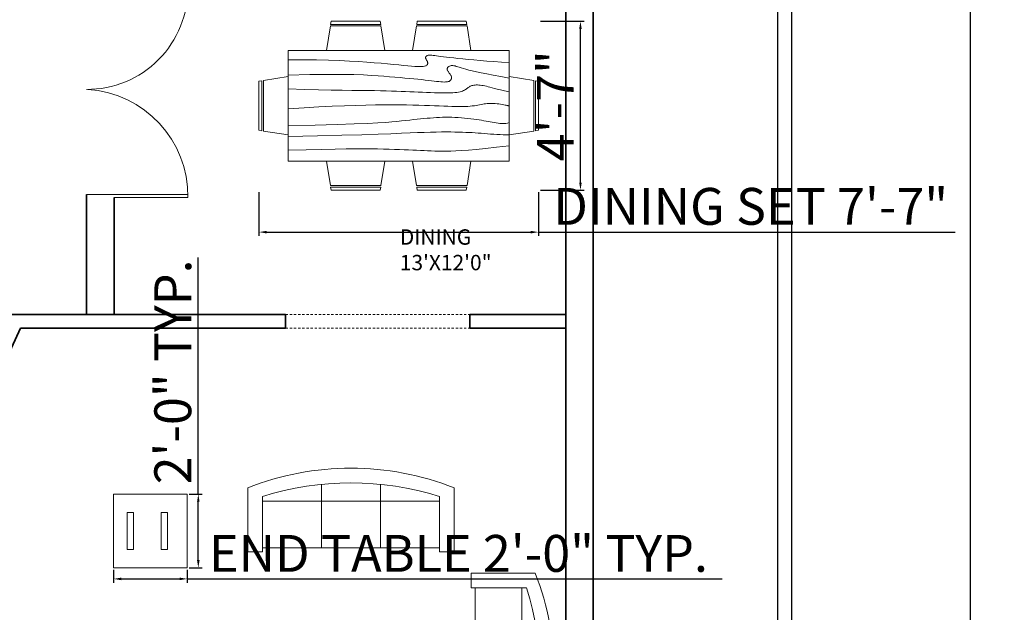
# Model space of a CAD drawing. Units: inches. Extents: x 2562 to 3392, y 1021 to 2243.
# Tile 4 of 6: x 2986 to 3306, y 1472 to 1665. Entities that reach past the tile are written whole.
import ezdxf

# ---------------------------------------------------------------- set-up
doc = ezdxf.new("R2010")
doc.units = ezdxf.units.IN
doc.linetypes.add('JIS_02_0.7', pattern=[1.35, 0.75, -0.6])
for name, color, linetype, lineweight in [('A-ANNO-DIMS', 2, 'Continuous', 18), ('A-AREA-IDEN', 7, 'Continuous', 18), ('A-DOOR', 4, 'Continuous', 18), ('A-FURN', 8, 'Continuous', 18), ('A-WALL', 7, 'Continuous', 35), ('A-WALL-HIDN', 7, 'JIS_02_0.7', 18), ('C-PROP', 7, 'Continuous', 30)]:
    doc.layers.add(name, color=color, linetype=linetype, lineweight=lineweight)
doc.styles.get("Standard").update_dxf_attribs({"font": 'arial.ttf'})
doc.dimstyles.new('ISO-25', dxfattribs={"dimtxt": 12, "dimasz": 2.5, "dimexe": 1.25, "dimexo": 0.625, "dimtad": 1, "dimdec": 1, "dimlunit": 3, "dimtxsty": 'Standard', "dimcen": 2.5, "dimadec": 0, "dimazin": 0, "dimtfac": 1, "dimtdec": 1, "dimtmove": 0, "dimatfit": 3, "dimfxl": 1, "dimarcsym": 0})

# ---------------------------------------------------------------- blocks, each defined once
blk = doc.blocks.new('Dining Set - 36 x 72 in.')
for p, q in [((-22.2343, 26.00059), (-23.4847, 17.99762)), ((-22.2304, 26), (-5.7608, 26)), ((-22, 27.5), (-22.1562, 26.50042)), ((-5.8416, 26.5), (-22.1534, 26.5)), ((-22, 27.5), (-6, 27.5)), ((-5.8437, 26.49966), (-6, 27.5)), ((-4.5152, 17.99762), (-5.7655, 25.99926)), ((5.7657, 26.00059), (4.5153, 17.99762)), ((5.7696, 26), (22.2392, 26)), ((6, 27.5), (5.8438, 26.50042)), ((22.1584, 26.5), (5.8466, 26.5)), ((6, 27.5), (22, 27.5)), ((22.1563, 26.49966), (22, 27.5)), ((23.4848, 17.99762), (22.2345, 25.99926)), ((36, 18), (-36, 18)), ((-36, 18), (-36, -18)), ((36, -18), (36, 18)), ((-45.5, 8), (-44.5004, 8.15617)), ((-45.5, 8), (-45.5, -8)), ((-44.5, -8.15843), (-44.5, 8.15338)), ((-44.0006, 8.23428), (-35.9976, 9.48474)), ((-44, 8.23041), (-44, -8.23915)), ((44.0006, 8.23428), (35.9976, 9.48474)), ((44, 8.23041), (44, -8.23915)), ((44.5, -8.15843), (44.5, 8.15338)), ((45.5, 8), (44.5005, 8.15617)), ((45.5, 8), (45.5, -8)), ((-44.4997, -8.15631), (-45.5, -8)), ((-35.9976, -9.48476), (-43.9993, -8.2345)), ((35.9976, -9.48476), (43.9993, -8.2345)), ((44.4997, -8.15631), (45.5, -8)), ((-36, -18), (36, -18)), ((-22.2343, -26.0006), (-23.4847, -17.99762)), ((-4.5152, -17.99762), (-5.7655, -25.99928)), ((5.7657, -26.0006), (4.5153, -17.99762)), ((23.4848, -17.99762), (22.2345, -25.99928)), ((-22.2304, -26), (-5.7608, -26)), ((-22, -27.5), (-22.1562, -26.50044)), ((-5.8416, -26.5), (-22.1534, -26.5)), ((-22, -27.5), (-6, -27.5)), ((-5.8437, -26.49967), (-6, -27.5)), ((5.7696, -26), (22.2392, -26)), ((6, -27.5), (5.8438, -26.50044)), ((22.1584, -26.5), (5.8466, -26.5)), ((6, -27.5), (22, -27.5)), ((22.1563, -26.49967), (22, -27.5))]:
    blk.add_line(p, q)
for points in [[(-36, 15), (-31.1772, 14.97754), (-26.8079, 14.91406), (-22.8538, 14.81543), (-19.276, 14.6875), (-16.0362, 14.53613), (-13.0957, 14.36718), (-10.4159, 14.18652), (-7.9583, 14), (-5.6904, 13.81315), (-3.6035, 13.63021), (-1.6954, 13.45508), (0.0365, 13.29166), (1.5945, 13.14388), (2.9811, 13.01562), (4.1988, 12.9108), (5.25, 12.83333), (6.1393, 12.78613), (6.8802, 12.76823), (7.4883, 12.77767), (7.9792, 12.8125), (8.3685, 12.87077), (8.6719, 12.95052), (8.9049, 13.0498), (9.0833, 13.16666), (9.2205, 13.29899), (9.3216, 13.44401), (9.3895, 13.59879), (9.4271, 13.76041), (9.4373, 13.92594), (9.4232, 14.09245), (9.3875, 14.257), (9.3333, 14.41666), (9.2638, 14.56917), (9.1836, 14.71484), (9.0975, 14.85465), (9.0104, 14.98958), (8.9272, 15.1206), (8.8529, 15.2487), (8.7922, 15.37483), (8.75, 15.5), (8.7305, 15.62467), (8.7344, 15.74739), (8.7617, 15.86621), (8.8125, 15.97916), (8.8867, 16.08431), (8.9844, 16.17968), (9.1055, 16.26334), (9.25, 16.33333), (9.4189, 16.38802), (9.6172, 16.42708), (9.8506, 16.45052), (10.125, 16.45833), (10.4463, 16.45052), (10.8203, 16.42708), (11.2529, 16.38802), (11.75, 16.33333), (12.3184, 16.26318), (12.9694, 16.17838), (13.7151, 16.07991), (14.5677, 15.96875), (15.5395, 15.84586), (16.6426, 15.71224), (17.8893, 15.56884), (19.2917, 15.41666), (20.859, 15.25667), (22.5879, 15.08984), (24.4721, 14.91715), (26.5052, 14.73958), (28.6809, 14.5581), (30.9929, 14.3737), (33.4347, 14.18733), (36, 14)], [(-36, 10), (-28.9766, 10.14274), (-23.1725, 10.20442), (-18.4241, 10.19775), (-14.5677, 10.13541), (-11.4399, 10.03011), (-8.877, 9.89453), (-6.7154, 9.74137), (-4.7917, 9.58333), (-2.9698, 9.43082), (-1.2246, 9.28515), (0.4415, 9.14534), (2.026, 9.01041), (3.5266, 8.87939), (4.9408, 8.7513), (6.266, 8.62516), (7.5, 8.5), (8.6411, 8.37549), (9.6914, 8.2539), (10.6538, 8.13818), (11.5312, 8.03125), (12.3267, 7.93603), (13.043, 7.85547), (13.6831, 7.79248), (14.25, 7.75), (14.7471, 7.7303), (15.1797, 7.73307), (15.5537, 7.75732), (15.875, 7.80208), (16.1494, 7.86637), (16.3828, 7.94922), (16.5811, 8.04964), (16.75, 8.16666), (16.8944, 8.29915), (17.0143, 8.44531), (17.1089, 8.60319), (17.1771, 8.77083), (17.218, 8.94629), (17.2305, 9.1276), (17.2137, 9.31282), (17.1667, 9.5), (17.0895, 9.6875), (16.987, 9.875), (16.8649, 10.0625), (16.7292, 10.25), (16.5856, 10.4375), (16.4401, 10.625), (16.2985, 10.8125), (16.1667, 11), (16.05, 11.18733), (15.9518, 11.3737), (15.8752, 11.5581), (15.8229, 11.73958), (15.798, 11.91715), (15.8034, 12.08984), (15.842, 12.25667), (15.9167, 12.41666), (16.0295, 12.56836), (16.1784, 12.70833), (16.3605, 12.83268), (16.5729, 12.9375), (16.8127, 13.01888), (17.0768, 13.07291), (17.3625, 13.0957), (17.6667, 13.08333), (17.9894, 13.03312), (18.3418, 12.94726), (18.7382, 12.82918), (19.1927, 12.68229), (19.7195, 12.51001), (20.3327, 12.31575), (21.0465, 12.10294), (21.875, 11.875), (22.8357, 11.63354), (23.959, 11.37304), (25.2786, 11.08618), (26.8282, 10.76562), (28.6414, 10.40405), (30.752, 9.99414), (33.1936, 9.52856), (36, 9)], [(-36, 5.5), (-30.7157, 5.3348), (-26.069, 5.20963), (-21.9946, 5.11767), (-18.4271, 5.05208), (-15.3009, 5.00602), (-12.5508, 4.97265), (-10.1112, 4.94515), (-7.9167, 4.91666), (-5.909, 4.88167), (-4.0586, 4.83984), (-2.3429, 4.79215), (-0.7396, 4.73958), (0.7739, 4.6831), (2.22, 4.6237), (3.6213, 4.56233), (5, 4.5), (6.373, 4.43782), (7.7344, 4.3776), (9.0723, 4.32129), (10.375, 4.27083), (11.6309, 4.22819), (12.8281, 4.19531), (13.9551, 4.17415), (15, 4.16666), (15.954, 4.17448), (16.819, 4.19791), (17.6001, 4.23698), (18.3021, 4.29166), (18.9299, 4.36198), (19.4883, 4.44791), (19.9823, 4.54948), (20.4167, 4.66666), (20.7969, 4.79899), (21.1302, 4.94401), (21.4245, 5.09879), (21.6875, 5.26041), (21.9271, 5.42594), (22.1511, 5.59245), (22.3672, 5.757), (22.5834, 5.91666), (22.8065, 6.06868), (23.0404, 6.21093), (23.2879, 6.34147), (23.5521, 6.45833), (23.8358, 6.55957), (24.142, 6.64323), (24.4735, 6.70735), (24.8334, 6.75), (25.2235, 6.76969), (25.642, 6.76692), (26.0858, 6.74267), (26.5521, 6.69791), (27.0379, 6.63362), (27.5404, 6.55078), (28.0565, 6.45036), (28.5834, 6.33333), (29.1242, 6.19987), (29.7071, 6.04687), (30.3661, 5.87044), (31.1354, 5.66666), (32.0493, 5.43164), (33.142, 5.16146), (34.4475, 4.85221), (36, 4.5)], [(-36, -1), (-30.7915, -0.6591), (-26.0195, -0.38216), (-21.6519, -0.16284), (-17.6563, 0.00521), (-14.0005, 0.12833), (-10.6523, 0.21289), (-7.5796, 0.26522), (-4.75, 0.29166), (-2.134, 0.29793), (0.2878, 0.28711), (2.5317, 0.26163), (4.6146, 0.22396), (6.5529, 0.17651), (8.3633, 0.12174), (10.0623, 0.06209), (11.6667, 0), (13.1899, -0.06201), (14.6341, -0.1211), (15.9982, -0.17432), (17.2813, -0.21875), (18.4823, -0.25147), (19.6003, -0.26953), (20.6343, -0.27002), (21.5834, -0.25), (22.4481, -0.20768), (23.2357, -0.14584), (23.9549, -0.06836), (24.6146, 0.02083), (25.2235, 0.11784), (25.7904, 0.21875), (26.3241, 0.31966), (26.8334, 0.41666), (27.3265, 0.50618), (27.8099, 0.58593), (28.2894, 0.65397), (28.7709, 0.70833), (29.2601, 0.74707), (29.763, 0.76823), (30.2855, 0.76985), (30.8334, 0.75), (31.4088, 0.70784), (31.9994, 0.64713), (32.589, 0.57275), (33.1615, 0.48958), (33.7008, 0.4025), (34.1908, 0.3164), (34.6153, 0.23616), (34.9584, 0.16666), (35.2099, 0.11165), (35.3848, 0.07031), (35.504, 0.04069), (35.5886, 0.02083), (35.6594, 0.00879), (35.7377, 0.0026), (35.8442, 0.00032), (36, 0)], [(-36, -6.5), (-27.1843, -6.31267), (-20.084, -6.1263), (-14.469, -5.9419), (-10.1094, -5.76042), (-6.7752, -5.58285), (-4.2363, -5.41016), (-2.2629, -5.24333), (-0.625, -5.08334), (0.8708, -4.93099), (2.2715, -4.78646), (3.5872, -4.64974), (4.8281, -4.52084), (6.0046, -4.39974), (7.127, -4.28646), (8.2053, -4.18099), (9.25, -4.08334), (10.2705, -3.99382), (11.2734, -3.91407), (12.2647, -3.84603), (13.25, -3.79167), (14.2354, -3.75293), (15.2266, -3.73177), (16.2295, -3.73015), (17.25, -3.75), (18.2912, -3.79248), (19.3451, -3.85547), (20.4009, -3.93604), (21.4479, -4.03125), (22.4754, -4.13819), (23.4727, -4.25391), (24.4289, -4.37549), (25.3334, -4.5), (26.1785, -4.62492), (26.9694, -4.74935), (27.7145, -4.87281), (28.4219, -4.99479), (29.1, -5.11483), (29.7572, -5.23242), (30.4016, -5.34709), (31.0417, -5.45834), (31.6837, -5.56437), (32.3262, -5.65821), (32.9658, -5.73153), (33.599, -5.77604), (34.2224, -5.78345), (34.8327, -5.74545), (35.4264, -5.65373), (36, -5.5)], [(-36, -10), (-26.4022, -9.81299), (-18.4675, -9.62891), (-11.9839, -9.45069), (-6.7396, -9.28125), (-2.5226, -9.12354), (0.8789, -8.98047), (3.6769, -8.85498), (6.0833, -8.75), (8.2767, -8.66765), (10.3021, -8.60677), (12.1712, -8.56543), (13.8958, -8.54167), (15.4876, -8.53353), (16.9583, -8.53907), (18.3197, -8.55632), (19.5834, -8.58334), (20.7616, -8.61841), (21.8685, -8.66081), (22.9188, -8.71004), (23.9271, -8.76563), (24.9081, -8.82707), (25.8763, -8.89388), (26.8465, -8.96558), (27.8334, -9.04167), (28.8474, -9.12118), (29.8828, -9.20117), (30.93, -9.27824), (31.9792, -9.34896), (33.0205, -9.40991), (34.0443, -9.45768), (35.0407, -9.48885), (36, -9.5)], [(-36, -14.5), (-30.0881, -14.33513), (-25.0332, -14.21224), (-20.7312, -14.12647), (-17.0781, -14.07292), (-13.97, -14.04671), (-11.3027, -14.04297), (-8.9724, -14.05681), (-6.875, -14.08334), (-4.9224, -14.11833), (-3.0905, -14.16016), (-1.3709, -14.20785), (0.2448, -14.26042), (1.7647, -14.3169), (3.1973, -14.3763), (4.5507, -14.43767), (5.8333, -14.5), (7.0554, -14.5621), (8.235, -14.62175), (9.3922, -14.67652), (10.5469, -14.72396), (11.7192, -14.76164), (12.929, -14.78711), (14.1965, -14.79794), (15.5417, -14.79167), (16.9933, -14.76424), (18.6152, -14.70508), (20.4804, -14.60197), (22.6615, -14.44271), (25.2312, -14.21509), (28.2624, -13.9069), (31.8277, -13.50594), (36, -13)]]:
    blk.add_lwpolyline(points)
blk = doc.blocks.new('Sofa - Roundback 7 ft.')
for p, q in [((-12.00002, -32.4421), (-12.00003, -6.5971)), ((11.99997, -32.4421), (11.99998, -6.5971)), ((-36.000027, -34), (-36.000027, -11.4696)), ((35.99998, -34), (35.99998, -11.4696)), ((-35.999844, -13.3819), (35.9998, -13.3819)), ((-36.000027, -32.4421), (35.99998, -32.4421))]:
    blk.add_line(p, q)
for points in [[(-36.000027, -34), (-42.000027, -34), (-42.000027, -8)], [(41.99998, -8), (41.99998, -34), (35.99998, -34)]]:
    blk.add_lwpolyline(points)
for centre, radius, start, end in [((0, -114.25), 114.25, 68.43141, 111.5686), ((-0.00001, -127.1968), 121.1968, 72.72033, 107.2797)]:
    blk.add_arc(centre, radius, start, end)
blk = doc.blocks.new('TABLE-END-24IN')
for p, q in [((0, 24), (24, 24)), ((0, 0), (0, 24)), ((24, 24), (24, 0)), ((4.5, 17.99), (6.5, 17.99)), ((4.5, 5.99), (4.5, 17.99)), ((6.5, 17.99), (6.5, 5.99)), ((15.56, 17.99), (17.56, 17.99)), ((15.56, 5.99), (15.56, 17.99)), ((17.56, 17.99), (17.56, 5.99)), ((6.5, 5.99), (4.5, 5.99)), ((17.56, 5.99), (15.56, 5.99)), ((24, 0), (0, 0))]:
    blk.add_line(p, q)
blk = doc.blocks.new('*D43')
at = {"layer": 'A-ANNO-DIMS', "color": 0, "lineweight": -2, "transparency": 16777216}
for p, q in [((3016.09, 1486), (3016.09, 1481.77)), ((3040.09, 1486), (3040.09, 1481.77)), ((3018.59, 1483.02), (3037.59, 1483.02)), ((3040.09, 1483.02), (3214.18, 1483.02))]:
    blk.add_line(p, q, dxfattribs=at)
at = {"layer": 'A-ANNO-DIMS', "color": 0, "transparency": 16777216}
for points in [[(3018.59, 1483.44), (3018.59, 1482.6), (3016.09, 1483.02)], [(3037.59, 1483.44), (3037.59, 1482.6), (3040.09, 1483.02)]]:
    blk.add_solid(points, dxfattribs=at)
at = {"layer": 'Defpoints', "color": 0, "transparency": 16777216}
for p in [(3016.09, 1486.62), (3040.09, 1486.62), (3040.09, 1483.02)]:
    blk.add_point(p, dxfattribs=at)
at = {"layer": 'A-ANNO-DIMS', "color": 0, "transparency": 16777216, "insert": (3128.38, 1489.77), "char_height": 12, "attachment_point": 5}
blk.add_mtext('END TABLE 2\'-0" TYP.', dxfattribs=at)
blk = doc.blocks.new('*D44')
at = {"layer": 'A-ANNO-DIMS', "color": 0, "lineweight": -2, "transparency": 16777216}
for p, q in [((3043.69, 1510.62), (3043.69, 1587.72)), ((3040.72, 1510.62), (3044.94, 1510.62)), ((3043.69, 1489.12), (3043.69, 1508.12)), ((3040.72, 1486.62), (3044.94, 1486.62))]:
    blk.add_line(p, q, dxfattribs=at)
at = {"layer": 'A-ANNO-DIMS', "color": 0, "transparency": 16777216}
for points in [[(3043.28, 1508.12), (3044.11, 1508.12), (3043.69, 1510.62)], [(3043.28, 1489.12), (3044.11, 1489.12), (3043.69, 1486.62)]]:
    blk.add_solid(points, dxfattribs=at)
at = {"layer": 'Defpoints', "color": 0, "transparency": 16777216}
for p in [(3040.09, 1510.62), (3043.69, 1510.62), (3040.09, 1486.62)]:
    blk.add_point(p, dxfattribs=at)
at = {"layer": 'A-ANNO-DIMS', "color": 0, "transparency": 16777216, "insert": (3036.94, 1550.42), "char_height": 12, "attachment_point": 5, "rotation": 90}
blk.add_mtext('2\'-0" TYP.', dxfattribs=at)
blk = doc.blocks.new('*D47')
at = {"layer": 'A-ANNO-DIMS', "color": 0, "lineweight": -2, "transparency": 16777216}
for p, q in [((3063.42, 1608.96), (3063.42, 1594.69)), ((3154.42, 1608.96), (3154.42, 1594.69)), ((3065.92, 1595.94), (3151.92, 1595.94)), ((3154.42, 1595.94), (3290.07, 1595.94))]:
    blk.add_line(p, q, dxfattribs=at)
at = {"layer": 'A-ANNO-DIMS', "color": 0, "transparency": 16777216}
for points in [[(3065.92, 1596.35), (3065.92, 1595.52), (3063.42, 1595.94)], [(3151.92, 1596.35), (3151.92, 1595.52), (3154.42, 1595.94)]]:
    blk.add_solid(points, dxfattribs=at)
at = {"layer": 'Defpoints', "color": 0, "transparency": 16777216}
for p in [(3063.42, 1609.59), (3154.42, 1609.59), (3154.42, 1595.94)]:
    blk.add_point(p, dxfattribs=at)
at = {"layer": 'A-ANNO-DIMS', "color": 0, "transparency": 16777216, "insert": (3223.49, 1602.77), "char_height": 12, "attachment_point": 5}
blk.add_mtext('DINING SET 7\'-7"', dxfattribs=at)
blk = doc.blocks.new('*D48')
at = {"layer": 'A-ANNO-DIMS', "color": 0, "lineweight": -2, "transparency": 16777216}
for p, q in [((3155.05, 1664.59), (3169.32, 1664.59)), ((3168.07, 1612.09), (3168.07, 1662.09)), ((3155.05, 1609.59), (3169.32, 1609.59))]:
    blk.add_line(p, q, dxfattribs=at)
at = {"layer": 'A-ANNO-DIMS', "color": 0, "transparency": 16777216}
for points in [[(3167.66, 1662.09), (3168.49, 1662.09), (3168.07, 1664.59)], [(3167.66, 1612.09), (3168.49, 1612.09), (3168.07, 1609.59)]]:
    blk.add_solid(points, dxfattribs=at)
at = {"layer": 'Defpoints', "color": 0, "transparency": 16777216}
for p in [(3154.42, 1664.59), (3168.07, 1664.59), (3154.42, 1609.59)]:
    blk.add_point(p, dxfattribs=at)
at = {"layer": 'A-ANNO-DIMS', "color": 0, "transparency": 16777216, "insert": (3161.45, 1637.09), "char_height": 12, "attachment_point": 5, "rotation": 90}
blk.add_mtext('4\'-7"', dxfattribs=at)
blk = doc.blocks.new('*D70')
at = {"layer": 'A-ANNO-DIMS', "color": 0, "lineweight": -2, "transparency": 16777216}
for p, q in [((3172.89, 2095.63), (3296.21, 2095.63)), ((3294.96, 2093.13), (3294.96, 1351.49)), ((3114.84, 1348.99), (3296.21, 1348.99))]:
    blk.add_line(p, q, dxfattribs=at)
at = {"layer": 'A-ANNO-DIMS', "color": 0, "transparency": 16777216}
for points in [[(3294.55, 2093.13), (3295.38, 2093.13), (3294.96, 2095.63)], [(3294.55, 1351.49), (3295.38, 1351.49), (3294.96, 1348.99)]]:
    blk.add_solid(points, dxfattribs=at)
at = {"layer": 'Defpoints', "color": 0, "transparency": 16777216}
for p in [(3172.26, 2095.63), (3114.22, 1348.99), (3294.96, 1348.99)]:
    blk.add_point(p, dxfattribs=at)
at = {"layer": 'A-ANNO-DIMS', "color": 0, "transparency": 16777216, "insert": (3288.13, 1722.31), "char_height": 12, "attachment_point": 5, "rotation": 90}
blk.add_mtext('62\'-2 1/2"', dxfattribs=at)

msp = doc.modelspace()

# ---------------------------------------------------------------- linework, layer by layer
at = {"layer": 'A-DOOR'}
for p, q in [((3007.26, 1608.23), (3016.26, 1608.23)), ((3016.26, 1608.23), (3040.26, 1608.23)), ((3040.26, 1607.23), (3016.26, 1607.23)), ((3040.26, 1608.23), (3040.26, 1607.23))]:
    msp.add_line(p, q, dxfattribs=at)
for centre, radius, start, end in [((3007.49, 1675.2), 32.78, 269.6005, 0.8741), ((3005.49, 1607.73), 34.77, 359.1761, 86.3317)]:
    msp.add_arc(centre, radius, start, end, dxfattribs=at)
at = {"layer": 'A-WALL'}
for p, q in [((3172.26, 2095.63), (3172.26, 1360.63)), ((3163.26, 2086.63), (3163.26, 1365.13)), ((3007.26, 1608.23), (3007.26, 1569.13)), ((3016.26, 1607.23), (3016.26, 1569.13)), ((2982.95, 1569.13), (3072.12, 1569.13)), ((3072.12, 1569.13), (3072.12, 1564.63)), ((3132.12, 1569.13), (3132.12, 1564.63)), ((3132.12, 1569.13), (3163.26, 1569.13)), ((2960.76, 1510.44), (2985.83, 1564.63)), ((2985.83, 1564.63), (3072.12, 1564.63)), ((3132.12, 1564.63), (3163.26, 1564.63))]:
    msp.add_line(p, q, dxfattribs=at)
at = {"layer": 'A-WALL-HIDN'}
for p, q in [((3072.12, 1569.13), (3132.12, 1569.13)), ((3072.12, 1564.63), (3132.12, 1564.63))]:
    msp.add_line(p, q, dxfattribs=at)
at = {"layer": 'C-PROP'}
for p, q in [((3236.76, 2160.13), (3236.76, 1080.13)), ((3232.26, 2155.63), (3232.26, 1084.63))]:
    msp.add_line(p, q, dxfattribs=at)

# ---------------------------------------------------------------- block references
at = {"layer": 'A-FURN'}
for name, p in [('Dining Set - 36 x 72 in.', (3108.92, 1637.09)), ('TABLE-END-24IN', (3016.09, 1486.62))]:
    msp.add_blockref(name, p, dxfattribs=at)
at = {"layer": 'A-FURN', "xscale": 0.8, "yscale": 0.8}
msp.add_blockref('Sofa - Roundback 7 ft.', (3093.38, 1519.06), dxfattribs=at)
at = {"layer": 'A-FURN', "xscale": 0.8, "yscale": 0.8, "rotation": 270}
msp.add_blockref('Sofa - Roundback 7 ft.', (3159.74, 1451.3), dxfattribs=at)

# ---------------------------------------------------------------- texts
at = {"layer": 'A-AREA-IDEN', "insert": (3109.28, 1596.85), "char_height": 5, "attachment_point": 1}
msp.add_mtext('DINING \\P13\'X12\'0"', dxfattribs=at)

# ---------------------------------------------------------------- dimensions: what is measured, and where the dimension line sits
at = {"layer": 'A-ANNO-DIMS'}
for base, p1, p2, picture, middle in [((3294.96, 1348.99), (3172.26, 2095.63), (3114.22, 1348.99), '*D70', (3288.13, 1722.31)), ((3168.07, 1664.59), (3154.42, 1609.59), (3154.42, 1664.59), '*D48', (3161.45, 1637.09))]:
    dim = msp.add_linear_dim(base=base, p1=p1, p2=p2, angle=90, dimstyle='ISO-25', override={"dimdec": 1, "dimlfac": 1, "dimrnd": 0, "dimzin": 1, "dimdsep": 46, "dimlunit": 4, "dimfrac": 2}, dxfattribs=at)
    dim.commit()
    dim.dimension.update_dxf_attribs({"geometry": picture, "text_midpoint": middle})
for base, p1, p2, text, picture, middle in [((3154.42, 1595.94), (3063.42, 1609.59), (3154.42, 1609.59), 'DINING SET <>', '*D47', (3223.49, 1602.77)), ((3040.09, 1483.02), (3016.09, 1486.62), (3040.09, 1486.62), 'END TABLE <> TYP.', '*D43', (3128.38, 1489.77))]:
    dim = msp.add_linear_dim(base=base, p1=p1, p2=p2, text=text, dimstyle='ISO-25', override={"dimdec": 1, "dimlfac": 1, "dimrnd": 0, "dimzin": 1, "dimdsep": 46, "dimlunit": 4, "dimfrac": 2}, dxfattribs=at)
    dim.commit()
    dim.dimension.update_dxf_attribs({"geometry": picture, "text_midpoint": middle})
dim = msp.add_linear_dim(base=(3043.69, 1510.62), p1=(3040.09, 1486.62), p2=(3040.09, 1510.62), angle=90, text='<> TYP.', dimstyle='ISO-25', override={"dimdec": 1, "dimlfac": 1, "dimrnd": 0, "dimzin": 1, "dimdsep": 46, "dimlunit": 4, "dimfrac": 2}, dxfattribs=at)
dim.commit()
dim.dimension.update_dxf_attribs({"geometry": '*D44', "text_midpoint": (3036.94, 1550.42)})

doc.saveas('drawing.dxf')
